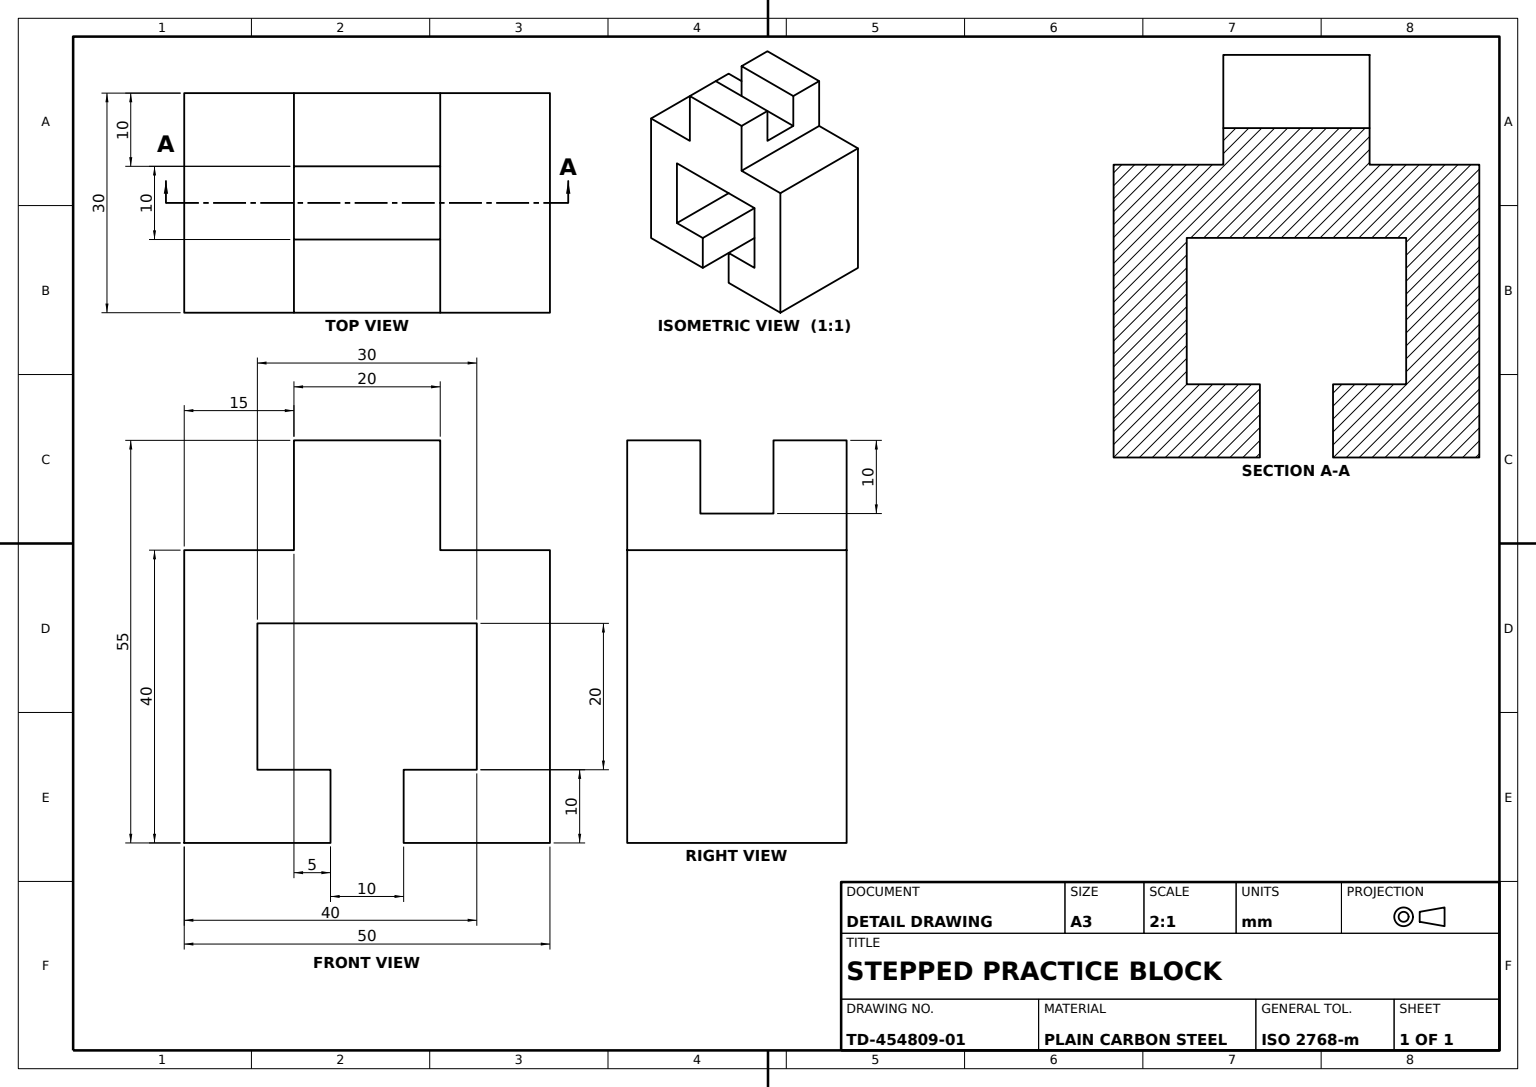
SolidWorks part; units mm, degrees
material "Plain Carbon Steel"
ref_plane "Front Plane" through (0, 0, 0) normal (0, 0, 1) x (1, 0, 0)
ref_plane "Top Plane" through (0, 0, 0) normal (0, 1, 0) x (1, 0, 0)
ref_plane "Right Plane" through (0, 0, 0) normal (1, 0, 0) x (0, 0, -1)
sketch "Block Profile Sketch" plane through (0, 0, 0) normal (0, 0, 1) x (1, 0, 0)
  line L0 (0, 0) -> (0, 40)
  line L1 (0, 40) -> (15, 40)
  line L2 (15, 40) -> (15, 55)
  line L3 (15, 55) -> (35, 55)
  line L4 (35, 55) -> (35, 40)
  line L5 (35, 40) -> (50, 40)
  line L6 (50, 40) -> (50, 0)
  line L7 (50, 0) -> (30, 0)
  line L8 (30, 0) -> (30, 10)
  line L9 (30, 10) -> (40, 10)
  line L10 (40, 10) -> (40, 30)
  line L11 (40, 30) -> (10, 30)
  line L12 (10, 30) -> (10, 10)
  line L13 (10, 10) -> (20, 10)
  line L14 (20, 10) -> (20, 0)
  line L15 (20, 0) -> (0, 0)
  dimension "D1" = 10
  dimension "D2" = 15
  dimension "D3" = 20
  dimension "D4" = 40
extrude "Block Body Extrude 30mm" add sketch "Block Profile Sketch" along normal blind 30
sketch "Pocket Sketch" plane through (0, 55, 0) normal (0, 1, 0) x (1, 0, 0)
  line L1 (15, -30) -> (15, 0) construction
  line L2 (15, -10) -> (35, -10)
  line L3 (35, -10) -> (35, -20)
  line L4 (35, -30) -> (35, 0) construction
  line L5 (35, -20) -> (15, -20)
  line L6 (35, 0) -> (15, 0) construction
  line L9 (15, -10) -> (15, -20)
  dimension "D1" = 10
  dimension "D2" = 20
extrude "Pocket Cut 10mm" cut sketch "Pocket Sketch" against normal blind 10
